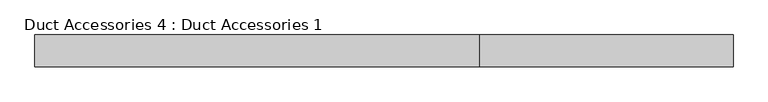
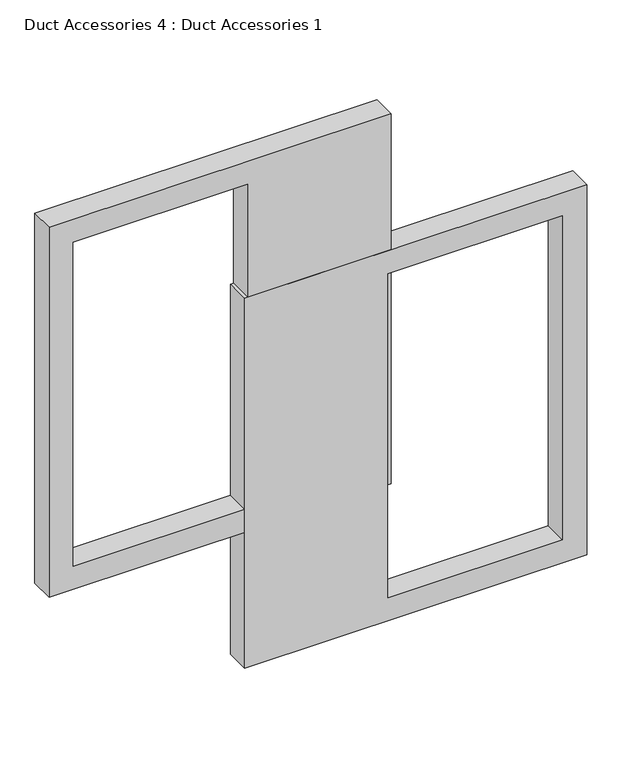
"""IFC4 building model written with IfcOpenShell, lengths in millimetres: damper geometry, Duct Accessories 4 : Duct Accessories 1."""

from ifc_helpers import new_model, si_unit, frame, origin, place, context, project, spatial, polyline, outline, extrude, source, transform, mapped, element, save


def duct_accessories_4_duct_accessories_1_42753040(model_context):
    return source(origin(), model_context, "Body", "SweptSolid", [
        extrude(outline(polyline([(28926.3403114, -12928.36893), (27707.1403114, -12928.36893), (27707.1403114, -11861.56893), (28926.3403114, -11861.56893), (28926.3403114, -12928.36893)]), holes=[polyline([(28850.1403114, -12480.9324751), (28850.1403114, -11937.76893), (27783.3403114, -11937.76893), (27783.3403114, -12480.9324751), (28850.1403114, -12480.9324751)])]), frame((0.0, -447.4934478, 0.0), z_axis=(0.0, 1.0, 0.0), x_axis=(0.0, 0.0, 1.0)), (0.0, 0.0, 1.0), 76.2),
        extrude(outline(polyline([(29373.7767663, -12471.5606701), (29373.7767663, -13538.3606701), (28154.5767663, -13538.3606701), (28154.5767663, -12471.5606701), (29373.7767663, -12471.5606701)]), holes=[polyline([(29297.5767663, -12918.997125), (28230.7767663, -12918.997125), (28230.7767663, -13462.1606701), (29297.5767663, -13462.1606701), (29297.5767663, -12918.997125)])]), frame((0.0, -447.4934478, 0.0), z_axis=(0.0, 1.0, 0.0), x_axis=(0.0, 0.0, 1.0)), (0.0, 0.0, 1.0), 76.2),
    ])


if __name__ == "__main__":
    model = new_model("IFC4")
    model_context = context("Model", 3, world=origin())
    ifc_project = project(units=[si_unit("LENGTHUNIT", "METRE", prefix="MILLI")], contexts=[model_context])
    site = spatial("IfcSite", under=ifc_project)
    building = spatial("IfcBuilding", under=site)
    placement = place(None, origin())
    duct_accessories_4_duct_accessories_1_shape = duct_accessories_4_duct_accessories_1_42753040(model_context)
    element("IfcDamper", 1, ObjectType="Duct Accessories 4 : Duct Accessories 1", at=placement, inside=building, context=model_context, shape_type="MappedRepresentation", body=[
        mapped(duct_accessories_4_duct_accessories_1_shape, transform((0.0, 0.0, 0.0), x_axis=(1.0, 0.0, 0.0), y_axis=(0.0, 1.0, 0.0), z_axis=(0.0, 0.0, 1.0))),
    ])
    save(model, "model.ifc")

# Revit data of these elements
# Element 1 (IfcDamper, "Duct Accessories 4 : Duct Accessories 1")
#   Materials on its faces: "border"
# Materials
#   "border": class "Generic", colour RGB 144 144 144, transparency 0, Cost = 0
